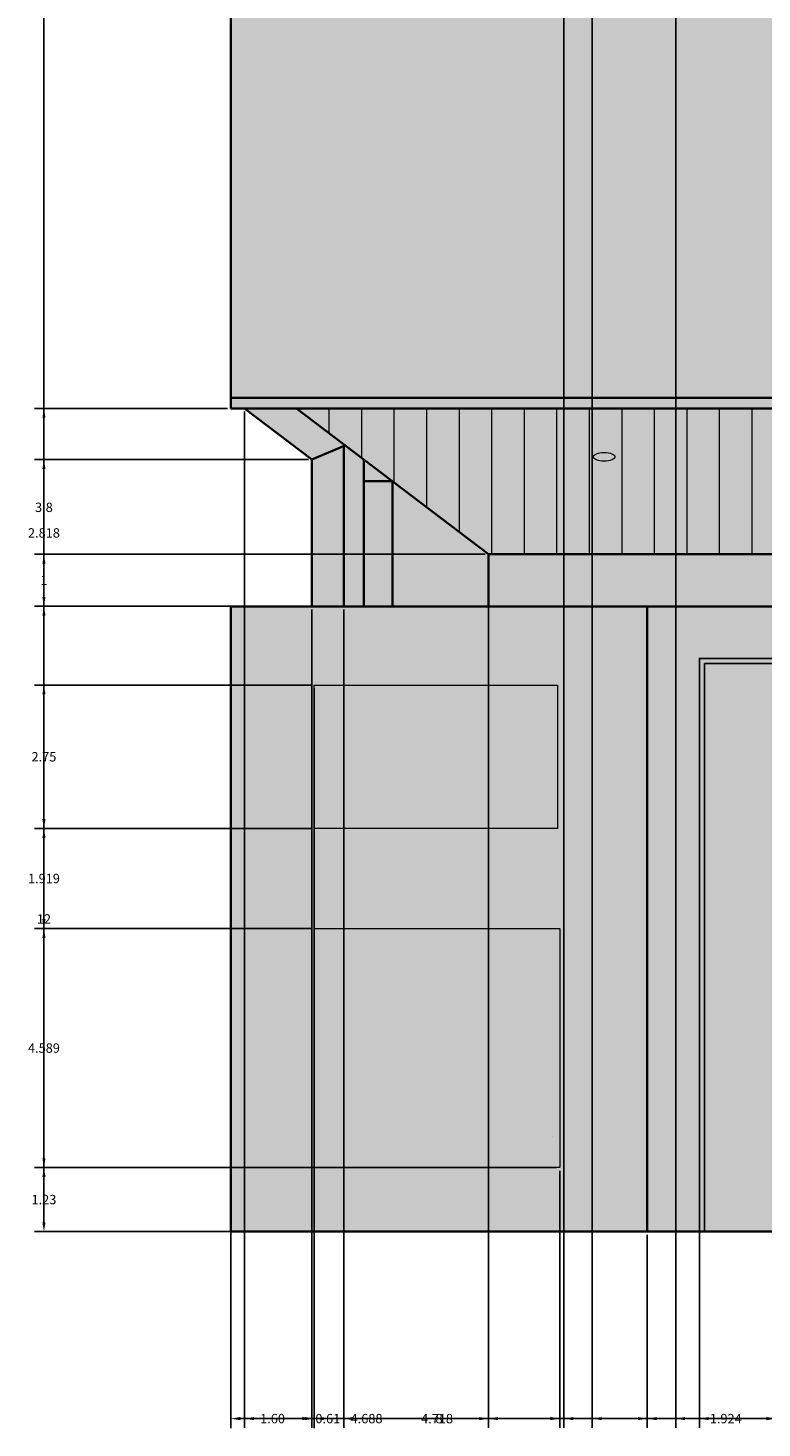
# Model space of a CAD drawing. Units: inches. Extents: x 18 to 59.8, y 2.7 to 81.2.
# Tile 1 of 9: x 18 to 32.1, y 2.7 to 29.5. Entities that reach past the tile are written whole.
import ezdxf

# ---------------------------------------------------------------- set-up
doc = ezdxf.new("R2010")
doc.units = ezdxf.units.IN
doc.header["$MEASUREMENT"] = 0
for name, color, linetype, lineweight in [('A-ANNO-DIMS', 2, 'Continuous', 18), ('A-DOOR', 3, 'Continuous', 25), ('A-ELEV', 7, 'Continuous', 35), ('A-ELEV-JALI', 9, 'Continuous', 18), ('A-ELEV-PATT', 8, 'Continuous', 13), ('E-LITE', 2, 'Continuous', 18)]:
    doc.layers.add(name, color=color, linetype=linetype, lineweight=lineweight)
doc.styles.get("Standard").update_dxf_attribs({"font": 'arial.ttf'})
doc.dimstyles.get("Standard").update_dxf_attribs({"dimtxt": 0.18, "dimasz": 0.18, "dimexe": 0.18, "dimexo": 0.0625, "dimgap": 0.09, "dimtad": 0, "dimtih": 1, "dimtoh": 1, "dimdec": 1, "dimzin": 0, "dimdsep": 46, "dimlunit": 3, "dimtxsty": 'Standard', "dimcen": 0.09, "dimadec": 0, "dimazin": 0, "dimtfac": 1, "dimtdec": 1, "dimtofl": 0, "dimtmove": 0, "dimatfit": 3, "dimfxl": 1, "dimtolj": 1, "dimtzin": 0, "dimarcsym": 0})

# ---------------------------------------------------------------- blocks, each defined once
blk = doc.blocks.new('LIGHT-SOFFIT-DOWN')
blk.add_ellipse((0.199, 0.085), major_axis=(0.207, 0), ratio=0.411448)
blk = doc.blocks.new('*D14')
at = {"layer": 'A-ANNO-DIMS', "color": 0, "lineweight": -2, "transparency": 16777216}
for p, q in [((21.797, 77.441), (18.09, 77.441)), ((18.27, 77.261), (18.27, 42.121)), ((18.27, 6.621), (18.27, 41.76)), ((21.797, 6.441), (18.09, 6.441))]:
    blk.add_line(p, q, dxfattribs=at)
at = {"layer": 'A-ANNO-DIMS', "color": 0, "transparency": 16777216}
for points in [[(18.24, 77.261), (18.3, 77.261), (18.27, 77.441)], [(18.24, 6.621), (18.3, 6.621), (18.27, 6.441)]]:
    blk.add_solid(points, dxfattribs=at)
at = {"layer": 'Defpoints', "color": 0, "transparency": 16777216}
for p in [(18.27, 77.441), (21.86, 77.441), (21.86, 6.441)]:
    blk.add_point(p, dxfattribs=at)
at = {"layer": 'A-ANNO-DIMS', "color": 0, "transparency": 16777216, "insert": (18.27, 41.941), "char_height": 0.18, "attachment_point": 5}
blk.add_mtext('\\A1;71', dxfattribs=at)
blk = doc.blocks.new('*D28')
at = {"layer": 'A-ANNO-DIMS', "color": 0, "lineweight": -2, "transparency": 16777216}
for p, q in [((21.86, 6.378), (21.86, 2.671)), ((29.86, 6.378), (29.86, 2.671)), ((22.04, 2.851), (25.711, 2.851)), ((29.68, 2.851), (26.009, 2.851))]:
    blk.add_line(p, q, dxfattribs=at)
at = {"layer": 'A-ANNO-DIMS', "color": 0, "transparency": 16777216}
for points in [[(22.04, 2.881), (22.04, 2.821), (21.86, 2.851)], [(29.68, 2.881), (29.68, 2.821), (29.86, 2.851)]]:
    blk.add_solid(points, dxfattribs=at)
at = {"layer": 'Defpoints', "color": 0, "transparency": 16777216}
for p in [(21.86, 6.441), (29.86, 6.441), (29.86, 2.851)]:
    blk.add_point(p, dxfattribs=at)
at = {"layer": 'A-ANNO-DIMS', "color": 0, "transparency": 16777216, "insert": (25.86, 2.851), "char_height": 0.18, "attachment_point": 5}
blk.add_mtext('\\A1;8', dxfattribs=at)
blk = doc.blocks.new('*D29')
at = {"layer": 'A-ANNO-DIMS', "color": 0, "lineweight": -2, "transparency": 16777216}
for p, q in [((29.86, 6.378), (29.86, 2.671)), ((47.86, 6.378), (47.86, 2.671)), ((30.04, 2.851), (38.649, 2.851)), ((47.68, 2.851), (39.071, 2.851))]:
    blk.add_line(p, q, dxfattribs=at)
at = {"layer": 'A-ANNO-DIMS', "color": 0, "transparency": 16777216}
for points in [[(30.04, 2.881), (30.04, 2.821), (29.86, 2.851)], [(47.68, 2.881), (47.68, 2.821), (47.86, 2.851)]]:
    blk.add_solid(points, dxfattribs=at)
at = {"layer": 'Defpoints', "color": 0, "transparency": 16777216}
for p in [(29.86, 6.441), (47.86, 6.441), (47.86, 2.851)]:
    blk.add_point(p, dxfattribs=at)
at = {"layer": 'A-ANNO-DIMS', "color": 0, "transparency": 16777216, "insert": (38.86, 2.851), "char_height": 0.18, "attachment_point": 5}
blk.add_mtext('\\A1;18', dxfattribs=at)
blk = doc.blocks.new('*D31')
at = {"layer": 'A-ANNO-DIMS', "color": 0, "lineweight": -2, "transparency": 16777216}
for p, q in [((21.859971, 18.378248), (21.859971, 2.670748)), ((23.462289, 16.867188), (23.462289, 2.670748)), ((22.039971, 2.850748), (22.34613, 2.850748)), ((23.282289, 2.850748), (22.97613, 2.850748))]:
    blk.add_line(p, q, dxfattribs=at)
at = {"layer": 'A-ANNO-DIMS', "color": 0, "transparency": 16777216}
for points in [[(22.039971, 2.880748), (22.039971, 2.820748), (21.859971, 2.850748)], [(23.282289, 2.880748), (23.282289, 2.820748), (23.462289, 2.850748)]]:
    blk.add_solid(points, dxfattribs=at)
at = {"layer": 'Defpoints', "color": 0, "transparency": 16777216}
for p in [(21.859971, 18.440748), (23.462289, 16.929688), (23.462289, 2.850748)]:
    blk.add_point(p, dxfattribs=at)
at = {"layer": 'A-ANNO-DIMS', "color": 0, "transparency": 16777216, "insert": (22.66113, 2.850748), "char_height": 0.18, "attachment_point": 5}
blk.add_mtext('\\A1;1.60', dxfattribs=at)
blk = doc.blocks.new('*D32')
at = {"layer": 'A-ANNO-DIMS', "color": 0, "lineweight": -2, "transparency": 16777216}
for p, q in [((23.462, 7.606), (23.462, 2.671)), ((28.18, 7.606), (28.18, 2.671)), ((23.642, 2.851), (25.424, 2.851)), ((28, 2.851), (26.219, 2.851))]:
    blk.add_line(p, q, dxfattribs=at)
at = {"layer": 'A-ANNO-DIMS', "color": 0, "transparency": 16777216}
for points in [[(23.642, 2.881), (23.642, 2.821), (23.462, 2.851)], [(28, 2.881), (28, 2.821), (28.18, 2.851)]]:
    blk.add_solid(points, dxfattribs=at)
at = {"layer": 'Defpoints', "color": 0, "transparency": 16777216}
for p in [(23.462, 7.669), (28.18, 7.669), (28.18, 2.851)]:
    blk.add_point(p, dxfattribs=at)
at = {"layer": 'A-ANNO-DIMS', "color": 0, "transparency": 16777216, "insert": (25.821, 2.851), "char_height": 0.18, "attachment_point": 5}
blk.add_mtext('\\A1;4.718', dxfattribs=at)
blk = doc.blocks.new('*D34')
at = {"layer": 'A-ANNO-DIMS', "color": 0, "lineweight": -2, "transparency": 16777216}
for p, q in [((30.86, 17.378), (30.86, 2.671)), ((46.86, 17.378), (46.86, 2.671)), ((31.04, 2.851), (38.65, 2.851)), ((46.68, 2.851), (39.07, 2.851))]:
    blk.add_line(p, q, dxfattribs=at)
at = {"layer": 'A-ANNO-DIMS', "color": 0, "transparency": 16777216}
for points in [[(31.04, 2.881), (31.04, 2.821), (30.86, 2.851)], [(46.68, 2.881), (46.68, 2.821), (46.86, 2.851)]]:
    blk.add_solid(points, dxfattribs=at)
at = {"layer": 'Defpoints', "color": 0, "transparency": 16777216}
for p in [(30.86, 17.441), (46.86, 17.441), (46.86, 2.851)]:
    blk.add_point(p, dxfattribs=at)
at = {"layer": 'A-ANNO-DIMS', "color": 0, "transparency": 16777216, "insert": (38.86, 2.851), "char_height": 0.18, "attachment_point": 5}
blk.add_mtext('\\A1;16', dxfattribs=at)
blk = doc.blocks.new('*D35')
at = {"layer": 'A-ANNO-DIMS', "color": 0, "lineweight": -2, "transparency": 16777216}
for p, q in [((21.797, 18.441), (18.09, 18.441)), ((18.27, 18.261), (18.27, 12.621)), ((18.27, 6.621), (18.27, 12.26)), ((21.797, 6.441), (18.09, 6.441))]:
    blk.add_line(p, q, dxfattribs=at)
at = {"layer": 'A-ANNO-DIMS', "color": 0, "transparency": 16777216}
for points in [[(18.24, 18.261), (18.3, 18.261), (18.27, 18.441)], [(18.24, 6.621), (18.3, 6.621), (18.27, 6.441)]]:
    blk.add_solid(points, dxfattribs=at)
at = {"layer": 'Defpoints', "color": 0, "transparency": 16777216}
for p in [(18.27, 18.441), (21.86, 18.441), (21.86, 6.441)]:
    blk.add_point(p, dxfattribs=at)
at = {"layer": 'A-ANNO-DIMS', "color": 0, "transparency": 16777216, "insert": (18.27, 12.441), "char_height": 0.18, "attachment_point": 5}
blk.add_mtext('\\A1;12', dxfattribs=at)
blk = doc.blocks.new('*D36')
at = {"layer": 'A-ANNO-DIMS', "color": 0, "lineweight": -2, "transparency": 16777216}
for p, q in [((21.797, 22.241), (18.09, 22.241)), ((18.27, 22.061), (18.27, 20.523)), ((18.27, 18.621), (18.27, 20.159)), ((21.797, 18.441), (18.09, 18.441))]:
    blk.add_line(p, q, dxfattribs=at)
at = {"layer": 'A-ANNO-DIMS', "color": 0, "transparency": 16777216}
for points in [[(18.24, 22.061), (18.3, 22.061), (18.27, 22.241)], [(18.24, 18.621), (18.3, 18.621), (18.27, 18.441)]]:
    blk.add_solid(points, dxfattribs=at)
at = {"layer": 'Defpoints', "color": 0, "transparency": 16777216}
for p in [(18.27, 22.241), (21.86, 22.241), (21.86, 18.441)]:
    blk.add_point(p, dxfattribs=at)
at = {"layer": 'A-ANNO-DIMS', "color": 0, "transparency": 16777216, "insert": (18.27, 20.341), "char_height": 0.18, "attachment_point": 5}
blk.add_mtext('\\A1;3.8', dxfattribs=at)
blk = doc.blocks.new('*D37')
at = {"layer": 'A-ANNO-DIMS', "color": 0, "lineweight": -2, "transparency": 16777216}
for p, q in [((28.117, 7.669), (18.09, 7.669)), ((18.27, 7.489), (18.27, 7.237)), ((18.27, 6.621), (18.27, 6.873)), ((29.797, 6.441), (18.09, 6.441))]:
    blk.add_line(p, q, dxfattribs=at)
at = {"layer": 'A-ANNO-DIMS', "color": 0, "transparency": 16777216}
for points in [[(18.24, 7.489), (18.3, 7.489), (18.27, 7.669)], [(18.24, 6.621), (18.3, 6.621), (18.27, 6.441)]]:
    blk.add_solid(points, dxfattribs=at)
at = {"layer": 'Defpoints', "color": 0, "transparency": 16777216}
for p in [(18.27, 7.669), (28.18, 7.669), (29.86, 6.441)]:
    blk.add_point(p, dxfattribs=at)
at = {"layer": 'A-ANNO-DIMS', "color": 0, "transparency": 16777216, "insert": (18.27, 7.055), "char_height": 0.18, "attachment_point": 5}
blk.add_mtext('\\A1;1.23', dxfattribs=at)
blk = doc.blocks.new('*D38')
at = {"layer": 'A-ANNO-DIMS', "color": 0, "lineweight": -2, "transparency": 16777216}
for p, q in [((23.4, 12.257), (18.09, 12.257)), ((18.27, 12.077), (18.27, 10.145)), ((18.27, 7.849), (18.27, 9.781)), ((23.4, 7.669), (18.09, 7.669))]:
    blk.add_line(p, q, dxfattribs=at)
at = {"layer": 'A-ANNO-DIMS', "color": 0, "transparency": 16777216}
for points in [[(18.24, 12.077), (18.3, 12.077), (18.27, 12.257)], [(18.24, 7.849), (18.3, 7.849), (18.27, 7.669)]]:
    blk.add_solid(points, dxfattribs=at)
at = {"layer": 'Defpoints', "color": 0, "transparency": 16777216}
for p in [(18.27, 12.257), (23.462, 12.257), (23.462, 7.669)]:
    blk.add_point(p, dxfattribs=at)
at = {"layer": 'A-ANNO-DIMS', "color": 0, "transparency": 16777216, "insert": (18.27, 9.963), "char_height": 0.18, "attachment_point": 5}
blk.add_mtext('\\A1;4.589', dxfattribs=at)
blk = doc.blocks.new('*D39')
at = {"layer": 'A-ANNO-DIMS', "color": 0, "lineweight": -2, "transparency": 16777216}
for p, q in [((23.4, 14.176), (18.09, 14.176)), ((18.27, 13.996), (18.27, 13.399)), ((18.27, 12.437), (18.27, 13.035)), ((23.4, 12.257), (18.09, 12.257))]:
    blk.add_line(p, q, dxfattribs=at)
at = {"layer": 'A-ANNO-DIMS', "color": 0, "transparency": 16777216}
for points in [[(18.24, 13.996), (18.3, 13.996), (18.27, 14.176)], [(18.24, 12.437), (18.3, 12.437), (18.27, 12.257)]]:
    blk.add_solid(points, dxfattribs=at)
at = {"layer": 'Defpoints', "color": 0, "transparency": 16777216}
for p in [(18.27, 14.176), (23.462, 14.176), (23.462, 12.257)]:
    blk.add_point(p, dxfattribs=at)
at = {"layer": 'A-ANNO-DIMS', "color": 0, "transparency": 16777216, "insert": (18.27, 13.217), "char_height": 0.18, "attachment_point": 5}
blk.add_mtext('\\A1;1.919', dxfattribs=at)
blk = doc.blocks.new('*D40')
at = {"layer": 'A-ANNO-DIMS', "color": 0, "lineweight": -2, "transparency": 16777216}
for p, q in [((23.4, 16.93), (18.09, 16.93)), ((18.27, 16.75), (18.27, 15.735)), ((18.27, 14.356), (18.27, 15.371)), ((23.4, 14.176), (18.09, 14.176))]:
    blk.add_line(p, q, dxfattribs=at)
at = {"layer": 'A-ANNO-DIMS', "color": 0, "transparency": 16777216}
for points in [[(18.24, 16.75), (18.3, 16.75), (18.27, 16.93)], [(18.24, 14.356), (18.3, 14.356), (18.27, 14.176)]]:
    blk.add_solid(points, dxfattribs=at)
at = {"layer": 'Defpoints', "color": 0, "transparency": 16777216}
for p in [(18.27, 16.93), (23.462, 16.93), (23.462, 14.176)]:
    blk.add_point(p, dxfattribs=at)
at = {"layer": 'A-ANNO-DIMS', "color": 0, "transparency": 16777216, "insert": (18.27, 15.553), "char_height": 0.18, "attachment_point": 5}
blk.add_mtext('\\A1;2.75', dxfattribs=at)
blk = doc.blocks.new('*D45')
at = {"layer": 'A-ANNO-DIMS', "color": 0, "lineweight": -2, "transparency": 16777216}
for p, q in [((26.748, 19.441), (18.09, 19.441)), ((18.27, 19.261), (18.27, 19.121)), ((18.27, 18.621), (18.27, 18.76)), ((26.748, 18.441), (18.09, 18.441))]:
    blk.add_line(p, q, dxfattribs=at)
at = {"layer": 'A-ANNO-DIMS', "color": 0, "transparency": 16777216}
for points in [[(18.24, 19.261), (18.3, 19.261), (18.27, 19.441)], [(18.24, 18.621), (18.3, 18.621), (18.27, 18.441)]]:
    blk.add_solid(points, dxfattribs=at)
at = {"layer": 'Defpoints', "color": 0, "transparency": 16777216}
for p in [(18.27, 19.441), (26.811, 19.441), (26.811, 18.441)]:
    blk.add_point(p, dxfattribs=at)
at = {"layer": 'A-ANNO-DIMS', "color": 0, "transparency": 16777216, "insert": (18.27, 18.941), "char_height": 0.18, "attachment_point": 5}
blk.add_mtext('\\A1;1', dxfattribs=at)
blk = doc.blocks.new('*D46')
at = {"layer": 'A-ANNO-DIMS', "color": 0, "lineweight": -2, "transparency": 16777216}
for p, q in [((26.811, 19.378), (26.811, 2.671)), ((50.578, 19.378), (50.578, 2.671)), ((26.991, 2.851), (38.229, 2.851)), ((50.398, 2.851), (39.159, 2.851))]:
    blk.add_line(p, q, dxfattribs=at)
at = {"layer": 'A-ANNO-DIMS', "color": 0, "transparency": 16777216}
for points in [[(26.991, 2.881), (26.991, 2.821), (26.811, 2.851)], [(50.398, 2.881), (50.398, 2.821), (50.578, 2.851)]]:
    blk.add_solid(points, dxfattribs=at)
at = {"layer": 'Defpoints', "color": 0, "transparency": 16777216}
for p in [(26.811, 19.441), (50.578, 19.441), (50.578, 2.851)]:
    blk.add_point(p, dxfattribs=at)
at = {"layer": 'A-ANNO-DIMS', "color": 0, "transparency": 16777216, "insert": (38.694, 2.851), "char_height": 0.18, "attachment_point": 5}
blk.add_mtext('\\A1;23.767', dxfattribs=at)
blk = doc.blocks.new('*D47')
at = {"layer": 'A-ANNO-DIMS', "color": 0, "lineweight": -2, "transparency": 16777216}
for p, q in [((22.123, 22.178), (22.123, 2.671)), ((26.811, 19.378), (26.811, 2.671)), ((22.303, 2.851), (24.07, 2.851)), ((26.631, 2.851), (24.865, 2.851))]:
    blk.add_line(p, q, dxfattribs=at)
at = {"layer": 'A-ANNO-DIMS', "color": 0, "transparency": 16777216}
for points in [[(22.303, 2.881), (22.303, 2.821), (22.123, 2.851)], [(26.631, 2.881), (26.631, 2.821), (26.811, 2.851)]]:
    blk.add_solid(points, dxfattribs=at)
at = {"layer": 'Defpoints', "color": 0, "transparency": 16777216}
for p in [(22.123, 22.241), (26.811, 19.441), (26.811, 2.851)]:
    blk.add_point(p, dxfattribs=at)
at = {"layer": 'A-ANNO-DIMS', "color": 0, "transparency": 16777216, "insert": (24.467, 2.851), "char_height": 0.18, "attachment_point": 5}
blk.add_mtext('\\A1;4.688', dxfattribs=at)
blk = doc.blocks.new('*D48')
at = {"layer": 'A-ANNO-DIMS', "color": 0, "lineweight": -2, "transparency": 16777216}
for p, q in [((23.416, 18.378), (23.416, 2.671)), ((24.03, 18.378), (24.03, 2.671)), ((23.236, 2.851), (23.056, 2.851)), ((24.21, 2.851), (24.39, 2.851))]:
    blk.add_line(p, q, dxfattribs=at)
at = {"layer": 'A-ANNO-DIMS', "color": 0, "transparency": 16777216}
for points in [[(23.236, 2.881), (23.236, 2.821), (23.416, 2.851)], [(24.21, 2.881), (24.21, 2.821), (24.03, 2.851)]]:
    blk.add_solid(points, dxfattribs=at)
at = {"layer": 'Defpoints', "color": 0, "transparency": 16777216}
for p in [(23.416, 18.441), (24.03, 18.441), (24.03, 2.851)]:
    blk.add_point(p, dxfattribs=at)
at = {"layer": 'A-ANNO-DIMS', "color": 0, "transparency": 16777216, "insert": (23.723, 2.851), "char_height": 0.18, "attachment_point": 5}
blk.add_mtext('\\A1;0.61', dxfattribs=at)
blk = doc.blocks.new('*D49')
at = {"layer": 'A-ANNO-DIMS', "color": 0, "lineweight": -2, "transparency": 16777216}
for p, q in [((23.354, 21.259), (18.09, 21.259)), ((18.27, 21.079), (18.27, 20.032)), ((18.27, 18.621), (18.27, 19.668)), ((23.354, 18.441), (18.09, 18.441))]:
    blk.add_line(p, q, dxfattribs=at)
at = {"layer": 'A-ANNO-DIMS', "color": 0, "transparency": 16777216}
for points in [[(18.24, 21.079), (18.3, 21.079), (18.27, 21.259)], [(18.24, 18.621), (18.3, 18.621), (18.27, 18.441)]]:
    blk.add_solid(points, dxfattribs=at)
at = {"layer": 'Defpoints', "color": 0, "transparency": 16777216}
for p in [(18.27, 21.259), (23.416, 21.259), (23.416, 18.441)]:
    blk.add_point(p, dxfattribs=at)
at = {"layer": 'A-ANNO-DIMS', "color": 0, "transparency": 16777216, "insert": (18.27, 19.85), "char_height": 0.18, "attachment_point": 5}
blk.add_mtext('\\A1;2.818', dxfattribs=at)
blk = doc.blocks.new('*D54')
at = {"layer": 'A-ANNO-DIMS', "color": 0, "lineweight": -2, "transparency": 16777216}
for p, q in [((28.258, 33.771), (28.258, 2.671)), ((48.33, 33.352), (48.33, 2.671)), ((28.438, 2.851), (37.899, 2.851)), ((48.15, 2.851), (38.689, 2.851))]:
    blk.add_line(p, q, dxfattribs=at)
at = {"layer": 'A-ANNO-DIMS', "color": 0, "transparency": 16777216}
for points in [[(28.438, 2.881), (28.438, 2.821), (28.258, 2.851)], [(48.15, 2.881), (48.15, 2.821), (48.33, 2.851)]]:
    blk.add_solid(points, dxfattribs=at)
at = {"layer": 'Defpoints', "color": 0, "transparency": 16777216}
for p in [(28.258, 33.834), (48.33, 33.414), (48.33, 2.851)]:
    blk.add_point(p, dxfattribs=at)
at = {"layer": 'A-ANNO-DIMS', "color": 0, "transparency": 16777216, "insert": (38.294, 2.851), "char_height": 0.18, "attachment_point": 5}
blk.add_mtext('\\A1;20.07', dxfattribs=at)
blk = doc.blocks.new('*D56')
at = {"layer": 'A-ANNO-DIMS', "color": 0, "lineweight": -2, "transparency": 16777216}
for p, q in [((30.406, 31.378), (30.406, 2.671)), ((32.33, 31.378), (32.33, 2.671)), ((30.586, 2.851), (30.983, 2.851)), ((32.15, 2.851), (31.753, 2.851))]:
    blk.add_line(p, q, dxfattribs=at)
at = {"layer": 'A-ANNO-DIMS', "color": 0, "transparency": 16777216}
for points in [[(30.586, 2.881), (30.586, 2.821), (30.406, 2.851)], [(32.15, 2.881), (32.15, 2.821), (32.33, 2.851)]]:
    blk.add_solid(points, dxfattribs=at)
at = {"layer": 'Defpoints', "color": 0, "transparency": 16777216}
for p in [(30.406, 31.441), (32.33, 31.441), (32.33, 2.851)]:
    blk.add_point(p, dxfattribs=at)
at = {"layer": 'A-ANNO-DIMS', "color": 0, "transparency": 16777216, "insert": (31.368, 2.851), "char_height": 0.18, "attachment_point": 5}
blk.add_mtext('\\A1;1.924', dxfattribs=at)
blk = doc.blocks.new('*D66')
at = {"layer": 'A-ANNO-DIMS', "color": 0, "lineweight": -2, "transparency": 16777216}
for p, q in [((28.804, 51.378), (28.804, 2.671)), ((48.567, 51.179), (48.567, 2.671)), ((28.984, 2.851), (38.231, 2.851)), ((48.387, 2.851), (39.14, 2.851))]:
    blk.add_line(p, q, dxfattribs=at)
at = {"layer": 'A-ANNO-DIMS', "color": 0, "transparency": 16777216}
for points in [[(28.984, 2.881), (28.984, 2.821), (28.804, 2.851)], [(48.387, 2.881), (48.387, 2.821), (48.567, 2.851)]]:
    blk.add_solid(points, dxfattribs=at)
at = {"layer": 'Defpoints', "color": 0, "transparency": 16777216}
for p in [(28.804, 51.441), (48.567, 51.242), (48.567, 2.851)]:
    blk.add_point(p, dxfattribs=at)
at = {"layer": 'A-ANNO-DIMS', "color": 0, "transparency": 16777216, "insert": (38.685, 2.851), "char_height": 0.18, "attachment_point": 5}
blk.add_mtext('\\A1;19.764', dxfattribs=at)

msp = doc.modelspace()

# ---------------------------------------------------------------- hatches: boundary and pattern name
at = {"layer": 'A-ELEV-PATT'}
h = msp.add_hatch(color=256, dxfattribs=at)
h.set_gradient(color1=(255, 255, 255), color2=(199, 200, 202))
h.paths.add_polyline_path([(38.86, 75.4521, 0.4125527), (36.86, 77.4407), (21.86, 77.4407), (21.86, 22.4407), (22.86, 22.4407), (48.86, 22.4407), (48.86, 30.9234, 0.4074473), (48.3302, 31.4407), (30.4061, 31.4407, -0.7603989), (34.0116, 44.4407), (47.86, 44.4407, -0.4142136), (48.86, 43.4407), (48.86, 48.4407, 0.4142136), (47.86, 49.4407), (32.2338, 49.4407, -0.2243142), (27.8411, 52.8427, -0.8480129), (38.86, 61.4407)])
h.paths.add_polyline_path([(55.86, 77.4407), (54.86, 77.4407), (54.86, 22.2407), (55.86, 22.2407)])
h.paths.add_polyline_path([(54.86, 51.5407), (53.4401, 51.5407), (53.4401, 29.6407), (54.86, 29.6407)])
h.paths.add_polyline_path([(54.86, 61.4407), (53.4401, 57.4407), (53.4401, 51.6407), (54.86, 51.6407)])
h.paths.add_polyline_path([(54.86, 29.4407), (54.471, 29.4407), (54.471, 22.2407), (54.86, 22.2407)])
h.paths.add_polyline_path([(55.5745, 22.2407), (54.86, 22.2407), (54.5745, 22.2407), (53.9347, 21.7925), (54.5877, 21.5495)])
h.paths.add_polyline_path([(54.5991, 21.5452), (53.9443, 21.789), (53.9443, 18.4407), (54.5991, 18.4407)])
h.paths.add_polyline_path([(53.9443, 21.789), (53.9347, 21.7925), (53.5816, 21.5452), (53.5816, 18.4407), (53.9443, 18.4407)])
h.paths.add_polyline_path([(53.3648, 20.6928), (52.8956, 21.0646), (52.8956, 18.4407), (53.3648, 18.4407)])
h.paths.add_polyline_path([(52.8956, 21.0646), (50.5775, 19.4407), (50.5775, 18.4407), (52.8956, 18.4407)])
h.paths.add_polyline_path([(53.5816, 21.5452), (52.8956, 21.0646), (53.3648, 20.6928), (53.5816, 20.8447)])
h.paths.add_polyline_path([(26.8109, 19.4407), (24.9672, 20.8407), (24.9672, 18.4407), (26.8109, 18.4407)])
h.paths.add_polyline_path([(24.9672, 20.8407), (24.4165, 20.8427), (24.4165, 18.4407), (24.9672, 18.4407)])
h.paths.add_polyline_path([(24.4165, 20.8427), (24.4165, 21.2589), (24.0588, 21.5305), (24.0301, 21.5183), (24.0301, 18.4407), (24.4165, 18.4407)])
h.paths.add_polyline_path([(24.0301, 21.5183), (23.4165, 21.2589), (23.4165, 18.4407), (24.0301, 18.4407)])
h.paths.add_polyline_path([(24.0301, 21.5183), (24.0588, 21.5305), (23.1234, 22.2407), (22.1234, 22.2407), (23.4165, 21.2589)])
h.paths.add_polyline_path([(24.4165, 21.2589), (24.4165, 20.8427), (24.9672, 20.8407)])
h.paths.add_polyline_path([(47.86, 18.4407), (29.86, 18.4407), (29.86, 6.4407), (30.86, 6.4407), (30.86, 17.4407), (38.86, 17.4407), (46.86, 17.4407), (46.86, 6.4407), (47.86, 6.4407)])
h.paths.add_polyline_path([(54.5756, 15.215), (54.5756, 6.4407), (55.86, 6.4407), (55.86, 18.4407), (47.86, 18.4407), (47.86, 6.4407), (49.1482, 6.4407), (49.1482, 15.215, -1)])
h = msp.add_hatch(color=256, dxfattribs=at)
h.paths.add_polyline_path([(27.8411, 52.8427, -0.7443789), (36.86, 61.4407), (38.86, 61.4407, 0.8480129)])
h.paths.add_polyline_path([(47.86, 44.4407), (34.0116, 44.4407, 0.7603989), (30.4061, 31.4407, -0.7376246), (34.0116, 43.4407), (47.86, 43.4407, -0.4142136), (48.86, 42.4407), (48.86, 43.4407, 0.4142136)])
h.paths.add_polyline_path([(54.5756, 15.215), (54.5756, 6.4407), (55.86, 6.4407), (55.86, 18.4407), (47.86, 18.4407), (47.86, 6.4407), (49.1482, 6.4407), (49.1482, 15.215, -1)])
h.paths.add_polyline_path([(47.86, 18.4407), (29.86, 18.4407), (29.86, 6.4407), (30.86, 6.4407), (30.86, 17.4407), (38.86, 17.4407), (46.86, 17.4407), (46.86, 6.4407), (47.86, 6.4407)])
h.paths.add_polyline_path([(55.86, 77.4407), (54.86, 77.4407), (54.86, 22.2407), (55.86, 22.2407)])
h = msp.add_hatch(color=256, dxfattribs=at)
h.dxf.hatch_style = 1
h.paths.add_polyline_path([(54.86, 69.4407), (38.86, 69.4407), (38.86, 61.4407), (54.86, 61.4407)])
h.paths.add_polyline_path([(54.86, 61.4407), (38.86, 61.4407), (36.86, 61.4407, 0.443414), (27.6986, 58.4407), (48.86, 58.4407), (48.86, 57.4407), (53.4401, 57.4407)])
h.paths.add_polyline_path([(37.4994, 59.9399), (37.4994, 59.8198, -2.4106499), (37.1187, 59.8198), (37.1187, 59.9399)], flags=16)
h.paths.add_polyline_path([(42.6125, 59.8012), (42.6125, 59.9213), (42.9933, 59.9213), (42.9933, 59.8012, -2.4106499)], flags=16)
h.paths.add_polyline_path([(49.5965, 59.971), (49.5965, 60.091), (49.9773, 60.091), (49.9773, 59.971, -2.4106499)], flags=16)
h.paths.add_polyline_path([(44.4671, 57.0407), (32.6671, 57.0407), (32.6671, 56.0407), (44.4671, 56.0407)])
h.paths.add_polyline_path([(47.86, 43.4407), (46.86, 43.4407), (34.0116, 43.4407, 0.2012983), (29.3481, 41.4407), (47.86, 41.4407, 1)])
h.paths.add_polyline_path([(36.5542, 42.5145), (36.5542, 42.6346), (36.9349, 42.6346), (36.9349, 42.5145, -2.4106499)], flags=16)
h.paths.add_polyline_path([(42.939, 42.5402), (42.939, 42.6603), (43.3198, 42.6603), (43.3198, 42.5402, -2.4106499)], flags=16)
h.paths.add_polyline_path([(54.471, 29.4407), (48.86, 29.4407), (48.86, 22.2407), (54.471, 22.2407)])
h.paths.add_polyline_path([(54.5745, 22.2407), (23.1234, 22.2407), (26.8109, 19.4407), (50.5775, 19.4407)])
h.paths.add_polyline_path([(54.5756, 15.215, 1), (49.1482, 15.215), (49.1482, 6.4407), (54.5756, 6.4407)])
h.paths.add_polyline_path([(49.8323, 12.602), (49.8323, 9.1225), (49.6657, 9.1225), (49.6657, 12.602)], flags=16)
h = msp.add_hatch(dxfattribs=at)
h.set_pattern_fill('ANSI31', color=256, scale=5, angle=45, style=0)
h.paths.add_polyline_path([(54.86, 69.4407), (38.86, 69.4407), (38.86, 61.4407), (54.86, 61.4407)])
h.paths.add_polyline_path([(54.86, 61.4407), (38.86, 61.4407), (36.86, 61.4407, 0.443414), (27.6986, 58.4407), (48.86, 58.4407), (48.86, 57.4407), (53.4401, 57.4407)])
h.paths.add_polyline_path([(37.1661, 59.8577), (37.1187, 59.8577), (37.1187, 59.9399), (37.4994, 59.9399), (37.4994, 59.8577), (37.452, 59.8577, -3.476462)], flags=16)
h.paths.add_polyline_path([(42.66, 59.8391), (42.6125, 59.8391), (42.6125, 59.9213), (42.9933, 59.9213), (42.9933, 59.8391), (42.9458, 59.8391, -3.476462)], flags=16)
h.paths.add_polyline_path([(49.644, 60.0088), (49.5965, 60.0088), (49.5965, 60.091), (49.9773, 60.091), (49.9773, 60.0088), (49.9298, 60.0088, -3.476462)], flags=16)
h.paths.add_polyline_path([(44.4671, 57.0407), (32.6671, 57.0407), (32.6671, 56.0407), (44.4671, 56.0407)])
h.paths.add_polyline_path([(47.86, 43.4407), (46.86, 43.4407), (34.0116, 43.4407, 0.2012983), (29.3481, 41.4407), (47.86, 41.4407, 1)])
h.paths.add_polyline_path([(36.6016, 42.5524), (36.5542, 42.5524), (36.5542, 42.6346), (36.9349, 42.6346), (36.9349, 42.5524), (36.8875, 42.5524, -3.476462)], flags=16)
h.paths.add_polyline_path([(42.9865, 42.578), (42.939, 42.578), (42.939, 42.6603), (43.3198, 42.6603), (43.3198, 42.578), (43.2723, 42.578, -3.476462)], flags=16)
h.paths.add_polyline_path([(54.471, 29.4407), (48.86, 29.4407), (48.86, 22.2407), (54.471, 22.2407)])
h.paths.add_polyline_path([(54.5745, 22.2407), (23.1234, 22.2407), (26.8109, 19.4407), (50.5775, 19.4407)])
h.paths.add_polyline_path([(54.5756, 15.215, 1), (49.1482, 15.215), (49.1482, 6.4407), (54.5756, 6.4407)])
h.paths.add_polyline_path([(49.8323, 9.1225), (49.6657, 9.1225), (49.6657, 12.602), (49.8323, 12.602)], flags=16)
h = msp.add_hatch(color=256, dxfattribs=at)
h.paths.add_polyline_path([(36.8875, 42.5524), (36.6016, 42.5524, 3.476462)])
h.paths.add_polyline_path([(43.2723, 42.578), (42.9865, 42.578, 3.476462)])
h.paths.add_polyline_path([(37.452, 59.8577), (37.1661, 59.8577, 3.476462)])
h.paths.add_polyline_path([(42.9458, 59.8391), (42.66, 59.8391, 3.476462)])
h.paths.add_polyline_path([(49.9298, 60.0088), (49.644, 60.0088, 3.476462)])
edge = h.paths.add_edge_path()
edge.add_ellipse((29.0313, 21.3107), major_axis=(-0.2068, 0), ratio=0.411448, start_angle=0, end_angle=360)
edge = h.paths.add_edge_path()
edge.add_ellipse((32.5919, 20.2963), major_axis=(-0.2068, 0), ratio=0.411448, start_angle=0, end_angle=360)
edge = h.paths.add_edge_path()
edge.add_ellipse((35.5044, 21.3908), major_axis=(-0.2068, 0), ratio=0.411448, start_angle=0, end_angle=360)
edge = h.paths.add_edge_path()
edge.add_ellipse((39.3877, 20.1968), major_axis=(-0.2068, 0), ratio=0.411448, start_angle=0, end_angle=360)
edge = h.paths.add_edge_path()
edge.add_ellipse((43.271, 21.3659), major_axis=(-0.2068, 0), ratio=0.411448, start_angle=0, end_angle=360)
edge = h.paths.add_edge_path()
edge.add_ellipse((47.3535, 20.1471), major_axis=(-0.2068, 0), ratio=0.411448, start_angle=0, end_angle=360)
h = msp.add_hatch(color=256, dxfattribs=at)
h.paths.add_polyline_path([(38.86, 17.4407), (30.86, 17.4407), (30.86, 6.4407), (30.96, 6.4407), (30.96, 17.3407), (38.86, 17.3407)])
h.paths.add_polyline_path([(46.86, 17.4407), (38.86, 17.4407), (38.86, 17.3407), (46.76, 17.3407), (46.76, 6.4407), (46.86, 6.4407)])
h.paths.add_polyline_path([(49.8323, 12.602), (49.6657, 12.602), (49.6657, 9.1225), (49.8323, 9.1225)])
h.paths.add_polyline_path([(48.86, 22.4407), (21.86, 22.4407), (21.86, 22.2407), (48.86, 22.2407)])
h.paths.add_polyline_path([(54.86, 29.6407), (48.86, 29.6407), (48.86, 29.4407), (54.86, 29.4407)])
edge = h.paths.add_edge_path()
edge.add_spline(control_points=[(48.3302, 33.5345), (48.1229, 33.671), (47.9155, 33.8074), (47.6839, 33.8336)], knot_values=[0, 0, 0, 0, 0.7121901, 0.7121901, 0.7121901, 0.7121901], degree=3, periodic=0)
edge.add_line((47.6839, 33.8336), (28.2583, 33.8336))
edge.add_arc((34.0631, 36.8836), 6.5573, 207.71831, 208.7099)
edge.add_line((28.3119, 33.7336), (47.6238, 33.7336))
edge.add_spline(control_points=[(47.6238, 33.7336), (47.6461, 33.7341), (47.6685, 33.7345), (47.6905, 33.7336)], knot_values=[0, 0, 0, 0, 0.0667446, 0.0667446, 0.0667446, 0.0667446], degree=3, periodic=0)
edge.add_spline(control_points=[(47.6905, 33.7336), (47.7384, 33.7318), (47.7849, 33.7239), (47.8302, 33.7113)], knot_values=[0.570104, 0.570104, 0.570104, 0.570104, 0.7151116, 0.7151116, 0.7151116, 0.7151116], degree=3, periodic=0)
edge.add_spline(control_points=[(47.8302, 33.7113), (48.0085, 33.6616), (48.1694, 33.5378), (48.3302, 33.4141)], knot_values=[0, 0, 0, 0, 0.570104, 0.570104, 0.570104, 0.570104], degree=3, periodic=0)
edge.add_line((48.3302, 33.4141), (48.3302, 33.5345))
h = msp.add_hatch(color=256, dxfattribs=at)
h.paths.add_polyline_path([(38.86, 17.3407), (30.96, 17.3407), (30.96, 6.4407), (38.86, 6.4407)])
h.paths.add_polyline_path([(46.76, 17.3407), (38.86, 17.3407), (38.86, 6.4407), (46.76, 6.4407)])
h.paths.add_polyline_path([(50.5775, 19.4407), (26.8109, 19.4407), (26.8109, 18.4407), (50.5775, 18.4407)])
h = msp.add_hatch(color=256, dxfattribs=at)
h.paths.add_polyline_path([(29.86, 18.4407), (21.86, 18.4407), (21.86, 6.4407), (29.86, 6.4407)])
h.paths.add_polyline_path([(23.4623, 12.2574), (28.1799, 12.2574), (28.1799, 7.6686), (23.4623, 7.6686)], flags=0)
h.paths.add_polyline_path([(23.4623, 14.1764), (23.4623, 16.9297), (28.1382, 16.9297), (28.1382, 14.1764)], flags=16)
h.paths.add_polyline_path([(28.1382, 16.9297), (23.4623, 16.9297), (23.4623, 14.1764), (28.1382, 14.1764)], flags=16)
h.paths.add_polyline_path([(28.1799, 12.2574), (23.4623, 12.2574), (23.4623, 7.6686), (28.1799, 7.6686)], flags=16)
h = msp.add_hatch(dxfattribs=at)
h.set_pattern_fill('AR-CONC', color=256, scale=5.2, angle=45, style=0)
h.paths.add_polyline_path([(28.1382, 16.9297), (23.4623, 16.9297), (23.4623, 14.1764), (28.1382, 14.1764)])
h.paths.add_polyline_path([(28.1799, 12.2574), (23.4623, 12.2574), (23.4623, 7.6686), (28.1799, 7.6686)])
h = msp.add_hatch(dxfattribs=at)
h.set_pattern_fill('AR-CONC', color=256, scale=5.2, angle=45, style=0)
h.paths.add_polyline_path([(28.1382, 16.9297), (23.4623, 16.9297), (23.4623, 14.1764), (28.1382, 14.1764)])
h.paths.add_polyline_path([(28.1799, 12.2574), (23.4623, 12.2574), (23.4623, 7.6686), (28.1799, 7.6686)])

# ---------------------------------------------------------------- linework, layer by layer
at = {"layer": 'A-DOOR'}
for points in [[(46.86, 6.4407), (46.86, 17.4407), (38.86, 17.4407), (30.86, 17.4407), (30.86, 6.4407)], [(46.76, 6.4407), (46.76, 17.3407), (38.86, 17.3407), (30.96, 17.3407), (30.96, 6.4407)]]:
    msp.add_lwpolyline(points, dxfattribs=at)
at = {"layer": 'A-ELEV'}
for p, q in [((21.86, 22.2407), (21.86, 77.4407)), ((21.86, 22.4407), (48.86, 22.4407)), ((21.86, 22.4407), (22.86, 22.4407)), ((21.86, 22.2407), (55.86, 22.2407)), ((22.1234, 22.2407), (23.4165, 21.2589)), ((23.1234, 22.2407), (26.8109, 19.4407)), ((23.4165, 21.2589), (24.0588, 21.5305)), ((24.0301, 21.5183), (24.0301, 18.4407)), ((23.4165, 21.2589), (23.4165, 18.4407)), ((24.4165, 21.2589), (24.4165, 18.4407)), ((24.4165, 20.8427), (24.9672, 20.8407)), ((24.9672, 20.8407), (24.9672, 18.4407)), ((26.8109, 19.4407), (50.5775, 19.4407)), ((26.8109, 19.4407), (26.8109, 18.4407)), ((21.86, 6.4407), (21.86, 18.4407)), ((21.86, 18.4407), (55.86, 18.4407)), ((23.4165, 18.4407), (24.4165, 18.4407)), ((29.86, 18.4407), (29.86, 6.4407)), ((29.86, 18.4407), (29.86, 6.4407)), ((29.86, 6.4407), (21.86, 6.4407)), ((29.86, 6.4407), (47.86, 6.4407))]:
    msp.add_line(p, q, dxfattribs=at)
at = {"layer": 'A-ELEV-JALI'}
for points in [[(23.4623, 16.9297), (28.1382, 16.9297), (28.1382, 14.1764), (23.4623, 14.1764)], [(23.4623, 12.2574), (28.1799, 12.2574), (28.1799, 7.6686), (23.4623, 7.6686)]]:
    msp.add_lwpolyline(points, close=True, dxfattribs=at)

# ---------------------------------------------------------------- block references
at = {"layer": 'E-LITE', "rotation": 180}
msp.add_blockref('LIGHT-SOFFIT-DOWN', (29.2302, 21.3955), dxfattribs=at)

# ---------------------------------------------------------------- dimensions: what is measured, and where the dimension line sits
at = {"layer": 'A-ANNO-DIMS'}
for base, p1, p2, override, picture, middle in [((18.27, 77.4407), (21.86, 6.4407), (21.86, 77.4407), {"dimdec": 0, "dimlfac": 1, "dimrnd": 0, "dimzin": 0, "dimdsep": 46, "dimlunit": 2}, '*D14', (18.27, 41.9407)), ((18.27, 22.2407), (21.86, 18.4407), (21.86, 22.2407), {"dimdec": 1, "dimlfac": 1, "dimrnd": 0, "dimzin": 0, "dimdsep": 46, "dimlunit": 2}, '*D36', (18.27, 20.3407)), ((18.27, 21.2589), (23.4165, 18.4407), (23.4165, 21.2589), {"dimdec": 3, "dimlfac": 1, "dimrnd": 0, "dimzin": 0, "dimdsep": 46, "dimlunit": 2}, '*D49', (18.27, 19.8498)), ((18.27, 19.4407), (26.8109, 18.4407), (26.8109, 19.4407), {"dimdec": 0, "dimlfac": 1, "dimrnd": 0, "dimzin": 0, "dimdsep": 46, "dimlunit": 2}, '*D45', (18.27, 18.9407)), ((18.27, 18.4407), (21.86, 6.4407), (21.86, 18.4407), {"dimdec": 0, "dimlfac": 1, "dimrnd": 0, "dimzin": 0, "dimdsep": 46, "dimlunit": 2}, '*D35', (18.27, 12.4407)), ((18.27, 16.9297), (23.4623, 14.1764), (23.4623, 16.9297), {"dimdec": 2, "dimlfac": 1, "dimrnd": 0, "dimzin": 0, "dimdsep": 46, "dimlunit": 2}, '*D40', (18.27, 15.553)), ((18.27, 14.1764), (23.4623, 12.2574), (23.4623, 14.1764), {"dimdec": 3, "dimlfac": 1, "dimrnd": 0, "dimzin": 0, "dimdsep": 46, "dimlunit": 2}, '*D39', (18.27, 13.2169)), ((18.27, 12.2574), (23.4623, 7.6686), (23.4623, 12.2574), {"dimdec": 3, "dimlfac": 1, "dimrnd": 0, "dimzin": 0, "dimdsep": 46, "dimlunit": 2}, '*D38', (18.27, 9.963)), ((18.27, 7.6686), (29.86, 6.4407), (28.1799, 7.6686), {"dimdec": 2, "dimlfac": 1, "dimrnd": 0, "dimzin": 0, "dimdsep": 46, "dimlunit": 2}, '*D37', (18.27, 7.0547))]:
    dim = msp.add_linear_dim(base=base, p1=p1, p2=p2, angle=90, dimstyle='Standard', override=override, dxfattribs=at)
    dim.commit()
    dim.dimension.update_dxf_attribs({"geometry": picture, "text_midpoint": middle})
for base, p1, p2, override, picture, middle in [((48.5671, 2.8507), (28.8035, 51.4407), (48.5671, 51.2416), {"dimdec": 3, "dimlfac": 1, "dimrnd": 0, "dimzin": 0, "dimdsep": 46, "dimlunit": 2}, '*D66', (38.6853, 2.8507)), ((48.3302, 2.8507), (28.2583, 33.8336), (48.3302, 33.4141), {"dimdec": 2, "dimlfac": 1, "dimrnd": 0, "dimzin": 0, "dimdsep": 46, "dimlunit": 2}, '*D54', (38.2942, 2.8507)), ((32.3302, 2.8507), (30.4061, 31.4407), (32.3302, 31.4407), {"dimdec": 3, "dimlfac": 1, "dimrnd": 0, "dimzin": 0, "dimdsep": 46, "dimlunit": 2}, '*D56', (31.3682, 2.8507)), ((26.81094, 2.85075), (22.12337, 22.24075), (26.81094, 19.44075), {"dimdec": 3, "dimlfac": 1, "dimrnd": 0, "dimzin": 0, "dimdsep": 46, "dimlunit": 2}, '*D47', (24.46715, 2.85075)), ((50.5775, 2.8507), (26.8109, 19.4407), (50.5775, 19.4407), {"dimdec": 3, "dimlfac": 1, "dimrnd": 0, "dimzin": 0, "dimdsep": 46, "dimlunit": 2}, '*D46', (38.6942, 2.8507)), ((23.4623, 2.8507), (21.86, 18.4407), (23.4623, 16.9297), {"dimdec": 2, "dimlfac": 1, "dimrnd": 0, "dimzin": 0, "dimdsep": 46, "dimlunit": 2}, '*D31', (22.6611, 2.8507)), ((24.0301, 2.8507), (23.4165, 18.4407), (24.0301, 18.4407), {"dimdec": 2, "dimlfac": 1, "dimrnd": 0, "dimzin": 0, "dimdsep": 46, "dimlunit": 2}, '*D48', (23.7233, 2.8507)), ((46.86, 2.8507), (30.86, 17.4407), (46.86, 17.4407), {"dimdec": 0, "dimlfac": 1, "dimrnd": 0, "dimzin": 0, "dimdsep": 46, "dimlunit": 2}, '*D34', (38.86, 2.8507)), ((28.1799, 2.8507), (23.4623, 7.6686), (28.1799, 7.6686), {"dimdec": 3, "dimlfac": 1, "dimrnd": 0, "dimzin": 0, "dimdsep": 46, "dimlunit": 2}, '*D32', (25.8211, 2.8507)), ((29.86, 2.8507), (21.86, 6.4407), (29.86, 6.4407), {"dimdec": 0, "dimlfac": 1, "dimrnd": 0, "dimzin": 0, "dimdsep": 46, "dimlunit": 2}, '*D28', (25.86, 2.8507)), ((47.86, 2.8507), (29.86, 6.4407), (47.86, 6.4407), {"dimdec": 0, "dimlfac": 1, "dimrnd": 0, "dimzin": 0, "dimdsep": 46, "dimlunit": 2}, '*D29', (38.86, 2.8507))]:
    dim = msp.add_linear_dim(base=base, p1=p1, p2=p2, dimstyle='Standard', override=override, dxfattribs=at)
    dim.commit()
    dim.dimension.update_dxf_attribs({"geometry": picture, "text_midpoint": middle})

doc.saveas('drawing.dxf')
